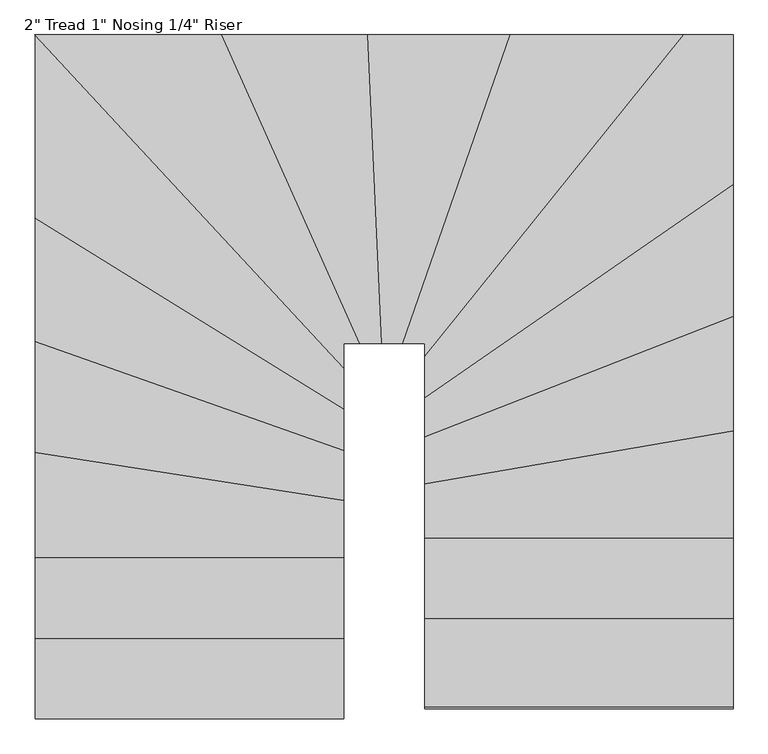
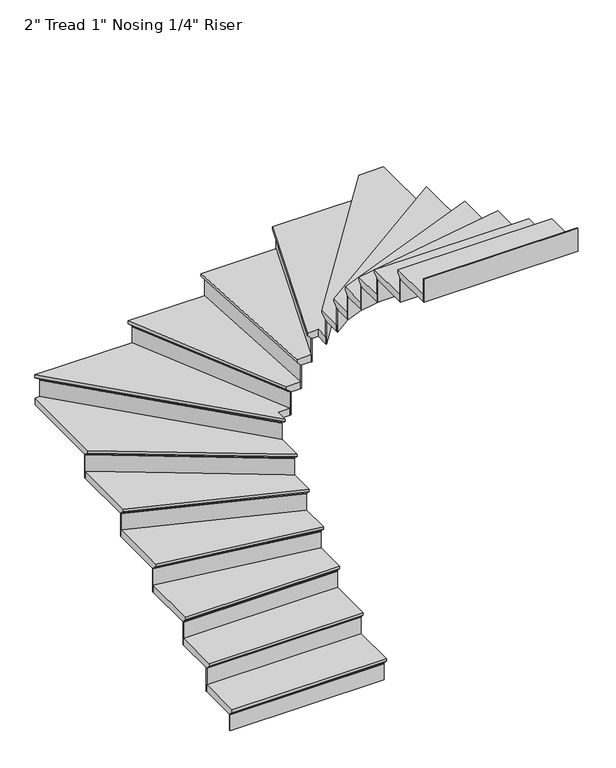
"""IFC4 building model written with IfcOpenShell, lengths in millimetres: stair flight geometry."""

from ifc_helpers import new_model, si_unit, origin, place, context, project, spatial, faceted_brep, source, transform, mapped, element, save


def stair_flight_3064df67(model_context):
    return source(origin(), model_context, "Body", "Brep", [
        faceted_brep([(-7275.2611447, 8794.085558, 319.6166667), (-7275.2611447, 8794.085558, 338.6666667), (-8342.0611447, 8794.085558, 338.6666667), (-8342.0611447, 8794.085558, 319.6166667), (-7275.2611447, 8819.485558, 294.2166667), (-8342.0611447, 8819.485558, 294.2166667), (-7275.2611447, 9098.885558, 338.6666667), (-8342.0611447, 9098.885558, 338.6666667), (-8342.0611447, 8819.485558, 287.8666667), (-8342.0611447, 9098.885558, 287.8666667), (-7275.2611447, 9098.885558, 287.8666667), (-7275.2611447, 8819.485558, 287.8666667)], [[[0, 1, 2, 3]], [[4, 0, 3, 5]], [[2, 1, 6, 7]], [[8, 9, 10, 11]], [[2, 7, 9, 8, 5, 3]], [[8, 11, 4, 5]], [[6, 1, 0, 4, 11, 10]], [[7, 6, 10, 9]]]),
        faceted_brep([(-7275.2611447, 8819.485558, 287.8666667), (-7275.2611447, 8819.485558, 169.3333333), (-7275.2611447, 8825.835558, 169.3333333), (-7275.2611447, 8825.835558, 287.8666667), (-8342.0611447, 8819.485558, 287.8666667), (-8342.0611447, 8825.835558, 287.8666667), (-8342.0611447, 8825.835558, 169.3333333), (-8342.0611447, 8819.485558, 169.3333333)], [[[0, 1, 2, 3]], [[4, 5, 6, 7]], [[1, 0, 4, 7]], [[2, 1, 7, 6]], [[3, 2, 6, 5]], [[0, 3, 5, 4]]]),
        faceted_brep([(-7275.2611447, 9098.885558, 457.2), (-7275.2611447, 9098.885558, 287.8666667), (-7275.2611447, 9105.235558, 287.8666667), (-7275.2611447, 9105.235558, 457.2), (-8342.0611447, 9098.885558, 457.2), (-8342.0611447, 9105.235558, 457.2), (-8342.0611447, 9105.235558, 287.8666667), (-8342.0611447, 9098.885558, 287.8666667)], [[[0, 1, 2, 3]], [[4, 5, 6, 7]], [[1, 0, 4, 7]], [[2, 1, 7, 6]], [[3, 2, 6, 5]], [[0, 3, 5, 4]]]),
        faceted_brep([(-8342.0611447, 9073.485558, 508.0), (-7275.2611447, 9073.485558, 508.0), (-7275.2611447, 9378.285558, 508.0), (-8342.0611447, 9378.285558, 508.0), (-8342.0611447, 9098.885558, 457.2), (-8342.0611447, 9378.285558, 457.2), (-7275.2611447, 9378.285558, 457.2), (-7275.2611447, 9098.885558, 457.2), (-8342.0611447, 9098.885558, 463.55), (-8342.0611447, 9073.485558, 488.95), (-7275.2611447, 9098.885558, 463.55), (-7275.2611447, 9073.485558, 488.95)], [[[0, 1, 2, 3]], [[4, 5, 6, 7]], [[0, 3, 5, 4, 8, 9]], [[4, 7, 10, 8]], [[2, 1, 11, 10, 7, 6]], [[3, 2, 6, 5]], [[11, 1, 0, 9]], [[10, 11, 9, 8]]]),
        faceted_brep([(-7275.2611447, 9378.285558, 626.5333333), (-7275.2611447, 9378.285558, 457.2), (-7275.2611447, 9384.635558, 457.2), (-7275.2611447, 9384.635558, 626.5333333), (-8342.0611447, 9378.285558, 626.5333333), (-8342.0611447, 9384.635558, 626.5333333), (-8342.0611447, 9384.635558, 457.2), (-8342.0611447, 9378.285558, 457.2)], [[[0, 1, 2, 3]], [[4, 5, 6, 7]], [[1, 0, 4, 7]], [[2, 1, 7, 6]], [[3, 2, 6, 5]], [[0, 3, 5, 4]]]),
        faceted_brep([(-8342.0611447, 9352.885558, 677.3333333), (-7275.2611447, 9352.885558, 677.3333333), (-7275.2611447, 9575.3066184, 677.3333333), (-8342.0611447, 9740.6711878, 677.3333333), (-8342.0611447, 9378.285558, 626.5333333), (-8342.0611447, 9740.6711878, 626.5333333), (-7275.2611447, 9575.3066184, 626.5333333), (-7275.2611447, 9378.285558, 626.5333333), (-8342.0611447, 9378.285558, 632.8833333), (-8342.0611447, 9352.885558, 658.2833333), (-7275.2611447, 9378.285558, 632.8833333), (-7275.2611447, 9352.885558, 658.2833333)], [[[0, 1, 2, 3]], [[4, 5, 6, 7]], [[0, 3, 5, 4, 8, 9]], [[4, 7, 10, 8]], [[2, 1, 11, 10, 7, 6]], [[3, 2, 6, 5]], [[11, 1, 0, 9]], [[10, 11, 9, 8]]]),
        faceted_brep([(-7275.2611447, 9575.3066184, 795.8666667), (-7275.2611447, 9575.3066184, 626.5333333), (-7275.2611447, 9581.7324547, 626.5333333), (-7275.2611447, 9581.7324547, 795.8666667), (-8342.0611447, 9740.6711878, 795.8666667), (-8342.0611447, 9747.0970241, 795.8666667), (-8342.0611447, 9747.0970241, 626.5333333), (-8342.0611447, 9740.6711878, 626.5333333)], [[[0, 1, 2, 3]], [[4, 5, 6, 7]], [[1, 0, 4, 7]], [[2, 1, 7, 6]], [[3, 2, 6, 5]], [[0, 3, 5, 4]]]),
        faceted_brep([(-8342.0611447, 9714.9678427, 846.6666667), (-7275.2611447, 9549.6032733, 846.6666667), (-7275.2611447, 9750.1745044, 846.6666667), (-8342.0611447, 10127.0738414, 846.6666667), (-8342.0611447, 9740.6711878, 795.8666667), (-8342.0611447, 10127.0738414, 795.8666667), (-7275.2611447, 9750.1745044, 795.8666667), (-7275.2611447, 9575.3066184, 795.8666667), (-8342.0611447, 9740.6711878, 802.2166667), (-8342.0611447, 9714.9678427, 827.6166667), (-7275.2611447, 9575.3066184, 802.2166667), (-7275.2611447, 9549.6032733, 827.6166667)], [[[0, 1, 2, 3]], [[4, 5, 6, 7]], [[0, 3, 5, 4, 8, 9]], [[4, 7, 10, 8]], [[2, 1, 11, 10, 7, 6]], [[3, 2, 6, 5]], [[11, 1, 0, 9]], [[10, 11, 9, 8]]]),
        faceted_brep([(-7275.2611447, 9750.1745044, 965.2), (-7275.2611447, 9750.1745044, 795.8666667), (-7275.2611447, 9756.9091582, 795.8666667), (-7275.2611447, 9756.9091582, 965.2), (-8342.0611447, 10127.0738414, 965.2), (-8342.0611447, 10133.8084951, 965.2), (-8342.0611447, 10133.8084951, 795.8666667), (-8342.0611447, 10127.0738414, 795.8666667)], [[[0, 1, 2, 3]], [[4, 5, 6, 7]], [[1, 0, 4, 7]], [[2, 1, 7, 6]], [[3, 2, 6, 5]], [[0, 3, 5, 4]]]),
        faceted_brep([(-8342.0611447, 10100.1352265, 1016.0), (-7275.2611447, 9723.2358895, 1016.0), (-7275.2611447, 9895.7459914, 1016.0), (-8342.0611447, 10557.0969884, 1016.0), (-8342.0611447, 10127.0738414, 965.2), (-8342.0611447, 10557.0969884, 965.2), (-7275.2611447, 9895.7459914, 965.2), (-7275.2611447, 9750.1745044, 965.2), (-8342.0611447, 10127.0738414, 971.55), (-8342.0611447, 10100.1352265, 996.95), (-7275.2611447, 9750.1745044, 971.55), (-7275.2611447, 9723.2358895, 996.95)], [[[0, 1, 2, 3]], [[4, 5, 6, 7]], [[0, 3, 5, 4, 8, 9]], [[4, 7, 10, 8]], [[2, 1, 11, 10, 7, 6]], [[3, 2, 6, 5]], [[11, 1, 0, 9]], [[10, 11, 9, 8]]]),
        faceted_brep([(-7275.2611447, 9895.7459914, 1134.5333333), (-7275.2611447, 9895.7459914, 965.2), (-7275.2611447, 9903.2172311, 965.2), (-7275.2611447, 9903.2172311, 1134.5333333), (-8342.0611447, 10557.0969884, 1134.5333333), (-8342.0611447, 10564.5682281, 1134.5333333), (-8342.0611447, 10564.5682281, 965.2), (-8342.0611447, 10557.0969884, 965.2)], [[[0, 1, 2, 3]], [[4, 5, 6, 7]], [[1, 0, 4, 7]], [[2, 1, 7, 6]], [[3, 2, 6, 5]], [[0, 3, 5, 4]]]),
        faceted_brep([(-8308.3760787, 11160.0172498, 1185.3333333), (-8342.0611447, 11160.0172498, 1185.3333333), (-8342.0611447, 10527.2120297, 1185.3333333), (-7275.2611447, 9865.8610326, 1185.3333333), (-7275.2611447, 10045.0066505, 1185.3333333), (-8342.0611447, 11160.0172498, 1134.5333333), (-8308.3760787, 11160.0172498, 1134.5333333), (-7275.2611447, 10045.0066505, 1134.5333333), (-7275.2611447, 9895.7459914, 1134.5333333), (-8342.0611447, 10557.0969884, 1134.5333333), (-7275.2611447, 9895.7459914, 1140.8833333), (-8342.0611447, 10557.0969884, 1140.8833333), (-7275.2611447, 9865.8610326, 1166.2833333), (-8342.0611447, 10527.2120297, 1166.2833333)], [[[0, 1, 2, 3, 4]], [[5, 6, 7, 8, 9]], [[1, 0, 6, 5]], [[9, 8, 10, 11]], [[4, 3, 12, 10, 8, 7]], [[0, 4, 7, 6]], [[12, 3, 2, 13]], [[10, 12, 13, 11]], [[2, 1, 5, 9, 11, 13]]]),
        faceted_brep([(-7275.2611447, 10045.0066505, 1303.8666667), (-7275.2611447, 10045.0066505, 1134.5333333), (-7275.2611447, 10054.3496243, 1134.5333333), (-7275.2611447, 10054.3496243, 1303.8666667), (-8308.3760787, 11160.0172498, 1303.8666667), (-8299.7193307, 11160.0172498, 1303.8666667), (-8299.7193307, 11160.0172498, 1134.5333333), (-8308.3760787, 11160.0172498, 1134.5333333)], [[[0, 1, 2, 3]], [[4, 5, 6, 7]], [[1, 0, 4, 7]], [[2, 1, 7, 6]], [[3, 2, 6, 5]], [[0, 3, 5, 4]]]),
        faceted_brep([(-8343.0030706, 11160.0172498, 1354.6666667), (-7275.2611447, 10007.6347554, 1354.6666667), (-7275.2611447, 10093.2172498, 1354.6666667), (-7192.6344871, 10093.2172498, 1354.6666667), (-7669.6752678, 11160.0172498, 1354.6666667), (-8308.3760787, 11160.0172498, 1303.8666667), (-7669.6752678, 11160.0172498, 1303.8666667), (-7192.6344871, 10093.2172498, 1303.8666667), (-7275.2611447, 10093.2172498, 1303.8666667), (-7275.2611447, 10045.0066505, 1303.8666667), (-8308.3760787, 11160.0172498, 1310.2166667), (-8343.0030706, 11160.0172498, 1335.6166667), (-7275.2611447, 10045.0066505, 1310.2166667), (-7275.2611447, 10007.6347554, 1335.6166667)], [[[0, 1, 2, 3, 4]], [[5, 6, 7, 8, 9]], [[0, 4, 6, 5, 10, 11]], [[5, 9, 12, 10]], [[2, 1, 13, 12, 9, 8]], [[3, 2, 8, 7]], [[4, 3, 7, 6]], [[13, 1, 0, 11]], [[12, 13, 11, 10]]]),
        faceted_brep([(-7192.6344871, 10093.2172498, 1473.2), (-7192.6344871, 10093.2172498, 1303.8666667), (-7185.6785241, 10093.2172498, 1303.8666667), (-7185.6785241, 10093.2172498, 1473.2), (-7669.6752678, 11160.0172498, 1473.2), (-7662.7193048, 11160.0172498, 1473.2), (-7662.7193048, 11160.0172498, 1303.8666667), (-7669.6752678, 11160.0172498, 1303.8666667)], [[[0, 1, 2, 3]], [[4, 5, 6, 7]], [[1, 0, 4, 7]], [[2, 1, 7, 6]], [[3, 2, 6, 5]], [[0, 3, 5, 4]]]),
        faceted_brep([(-7697.49912, 11160.0172498, 1524.0), (-7220.4583393, 10093.2172498, 1524.0), (-7118.6029726, 10093.2172498, 1524.0), (-7167.3410541, 11160.0172498, 1524.0), (-7669.6752678, 11160.0172498, 1473.2), (-7167.3410541, 11160.0172498, 1473.2), (-7118.6029726, 10093.2172498, 1473.2), (-7192.6344871, 10093.2172498, 1473.2), (-7669.6752678, 11160.0172498, 1479.55), (-7697.49912, 11160.0172498, 1504.95), (-7192.6344871, 10093.2172498, 1479.55), (-7220.4583393, 10093.2172498, 1504.95)], [[[0, 1, 2, 3]], [[4, 5, 6, 7]], [[0, 3, 5, 4, 8, 9]], [[4, 7, 10, 8]], [[3, 2, 6, 5]], [[11, 1, 0, 9]], [[10, 11, 9, 8]], [[2, 1, 11, 10, 7, 6]]]),
        faceted_brep([(-7118.6029726, 10093.2172498, 1642.5333333), (-7118.6029726, 10093.2172498, 1473.2), (-7112.2463491, 10093.2172498, 1473.2), (-7112.2463491, 10093.2172498, 1642.5333333), (-7167.3410541, 11160.0172498, 1642.5333333), (-7160.9844306, 11160.0172498, 1642.5333333), (-7160.9844306, 11160.0172498, 1473.2), (-7167.3410541, 11160.0172498, 1473.2)], [[[0, 1, 2, 3]], [[4, 5, 6, 7]], [[1, 0, 4, 7]], [[2, 1, 7, 6]], [[3, 2, 6, 5]], [[0, 3, 5, 4]]]),
        faceted_brep([(-7192.7675482, 11160.0172498, 1693.3333333), (-7144.0294667, 10093.2172498, 1693.3333333), (-7045.1202005, 10093.2172498, 1693.3333333), (-6671.9374808, 11160.0172498, 1693.3333333), (-7167.3410541, 11160.0172498, 1642.5333333), (-6671.9374808, 11160.0172498, 1642.5333333), (-7045.1202005, 10093.2172498, 1642.5333333), (-7118.6029726, 10093.2172498, 1642.5333333), (-7167.3410541, 11160.0172498, 1648.8833333), (-7192.7675482, 11160.0172498, 1674.2833333), (-7118.6029726, 10093.2172498, 1648.8833333), (-7144.0294667, 10093.2172498, 1674.2833333)], [[[0, 1, 2, 3]], [[4, 5, 6, 7]], [[0, 3, 5, 4, 8, 9]], [[4, 7, 10, 8]], [[2, 1, 11, 10, 7, 6]], [[3, 2, 6, 5]], [[11, 1, 0, 9]], [[10, 11, 9, 8]]]),
        faceted_brep([(-7045.1202005, 10093.2172498, 1811.8666667), (-7045.1202005, 10093.2172498, 1642.5333333), (-7038.3928839, 10093.2172498, 1642.5333333), (-7038.3928839, 10093.2172498, 1811.8666667), (-6671.9374808, 11160.0172498, 1811.8666667), (-6665.2101642, 11160.0172498, 1811.8666667), (-6665.2101642, 11160.0172498, 1642.5333333), (-6671.9374808, 11160.0172498, 1642.5333333)], [[[0, 1, 2, 3]], [[4, 5, 6, 7]], [[1, 0, 4, 7]], [[2, 1, 7, 6]], [[3, 2, 6, 5]], [[0, 3, 5, 4]]]),
        faceted_brep([(-6698.8467469, 11160.0172498, 1862.6666667), (-7072.0294667, 10093.2172498, 1862.6666667), (-6995.8611447, 10093.2172498, 1862.6666667), (-6995.8611447, 10007.4990501, 1862.6666667), (-6067.5072178, 11160.0172498, 1862.6666667), (-6671.9374808, 11160.0172498, 1811.8666667), (-6067.5072178, 11160.0172498, 1811.8666667), (-6995.8611447, 10007.4990501, 1811.8666667), (-6995.8611447, 10093.2172498, 1811.8666667), (-7045.1202005, 10093.2172498, 1811.8666667), (-6671.9374808, 11160.0172498, 1818.2166667), (-6698.8467469, 11160.0172498, 1843.6166667), (-7045.1202005, 10093.2172498, 1818.2166667), (-7072.0294667, 10093.2172498, 1843.6166667)], [[[0, 1, 2, 3, 4]], [[5, 6, 7, 8, 9]], [[0, 4, 6, 5, 10, 11]], [[5, 9, 12, 10]], [[2, 1, 13, 12, 9, 8]], [[3, 2, 8, 7]], [[4, 3, 7, 6]], [[13, 1, 0, 11]], [[12, 13, 11, 10]]]),
        faceted_brep([(-6995.8611447, 10007.4990501, 1981.2), (-6995.8611447, 10007.4990501, 1811.8666667), (-6995.8611447, 9997.3763585, 1811.8666667), (-6995.8611447, 9997.3763585, 1981.2), (-6067.5072178, 11160.0172498, 1981.2), (-6059.3533852, 11160.0172498, 1981.2), (-6059.3533852, 11160.0172498, 1811.8666667), (-6067.5072178, 11160.0172498, 1811.8666667)], [[[0, 1, 2, 3]], [[4, 5, 6, 7]], [[1, 0, 4, 7]], [[2, 1, 7, 6]], [[3, 2, 6, 5]], [[0, 3, 5, 4]]]),
        faceted_brep([(-5929.0611447, 10611.3875661, 2032.0), (-5929.0611447, 11160.0172498, 2032.0), (-6100.1225484, 11160.0172498, 2032.0), (-6995.8611447, 10047.9898167, 2032.0), (-6995.8611447, 9873.2783158, 2032.0), (-5929.0611447, 11160.0172498, 1981.2), (-5929.0611447, 10611.3875661, 1981.2), (-6995.8611447, 9873.2783158, 1981.2), (-6995.8611447, 10007.4990501, 1981.2), (-6067.5072178, 11160.0172498, 1981.2), (-6067.5072178, 11160.0172498, 1987.55), (-6100.1225484, 11160.0172498, 2012.95), (-6995.8611447, 10007.4990501, 1987.55), (-6995.8611447, 10047.9898167, 2012.95)], [[[0, 1, 2, 3, 4]], [[5, 6, 7, 8, 9]], [[1, 0, 6, 5]], [[2, 1, 5, 9, 10, 11]], [[9, 8, 12, 10]], [[4, 3, 13, 12, 8, 7]], [[0, 4, 7, 6]], [[13, 3, 2, 11]], [[12, 13, 11, 10]]]),
        faceted_brep([(-6995.8611447, 9873.2783158, 2150.5333333), (-6995.8611447, 9873.2783158, 1981.2), (-6995.8611447, 9865.5565668, 1981.2), (-6995.8611447, 9865.5565668, 2150.5333333), (-5929.0611447, 10611.3875661, 2150.5333333), (-5929.0611447, 10603.6658171, 2150.5333333), (-5929.0611447, 10603.6658171, 1981.2), (-5929.0611447, 10611.3875661, 1981.2)], [[[0, 1, 2, 3]], [[4, 5, 6, 7]], [[1, 0, 4, 7]], [[2, 1, 7, 6]], [[3, 2, 6, 5]], [[0, 3, 5, 4]]]),
        faceted_brep([(-5929.0611447, 10642.2745621, 2201.3333333), (-6995.8611447, 9904.1653118, 2201.3333333), (-6995.8611447, 9741.7204172, 2201.3333333), (-5929.0611447, 10158.6104329, 2201.3333333), (-5929.0611447, 10611.3875661, 2150.5333333), (-5929.0611447, 10158.6104329, 2150.5333333), (-6995.8611447, 9741.7204172, 2150.5333333), (-6995.8611447, 9873.2783158, 2150.5333333), (-5929.0611447, 10611.3875661, 2156.8833333), (-5929.0611447, 10642.2745621, 2182.2833333), (-6995.8611447, 9873.2783158, 2156.8833333), (-6995.8611447, 9904.1653118, 2182.2833333)], [[[0, 1, 2, 3]], [[4, 5, 6, 7]], [[0, 3, 5, 4, 8, 9]], [[4, 7, 10, 8]], [[2, 1, 11, 10, 7, 6]], [[3, 2, 6, 5]], [[11, 1, 0, 9]], [[10, 11, 9, 8]]]),
        faceted_brep([(-6995.8611447, 9741.7204172, 2319.8666667), (-6995.8611447, 9741.7204172, 2150.5333333), (-6995.8611447, 9734.9027722, 2150.5333333), (-6995.8611447, 9734.9027722, 2319.8666667), (-5929.0611447, 10158.6104329, 2319.8666667), (-5929.0611447, 10151.7927879, 2319.8666667), (-5929.0611447, 10151.7927879, 2150.5333333), (-5929.0611447, 10158.6104329, 2150.5333333)], [[[0, 1, 2, 3]], [[4, 5, 6, 7]], [[1, 0, 4, 7]], [[2, 1, 7, 6]], [[3, 2, 6, 5]], [[0, 3, 5, 4]]]),
        faceted_brep([(-5929.0611447, 10185.881013, 2370.6666667), (-6995.8611447, 9768.9909973, 2370.6666667), (-6995.8611447, 9580.5364125, 2370.6666667), (-5929.0611447, 9763.9899323, 2370.6666667), (-5929.0611447, 10158.6104329, 2319.8666667), (-5929.0611447, 9763.9899323, 2319.8666667), (-6995.8611447, 9580.5364125, 2319.8666667), (-6995.8611447, 9741.7204172, 2319.8666667), (-5929.0611447, 10158.6104329, 2326.2166667), (-5929.0611447, 10185.881013, 2351.6166667), (-6995.8611447, 9741.7204172, 2326.2166667), (-6995.8611447, 9768.9909973, 2351.6166667)], [[[0, 1, 2, 3]], [[4, 5, 6, 7]], [[0, 3, 5, 4, 8, 9]], [[4, 7, 10, 8]], [[2, 1, 11, 10, 7, 6]], [[3, 2, 6, 5]], [[11, 1, 0, 9]], [[10, 11, 9, 8]]]),
        faceted_brep([(-6995.8611447, 9580.5364125, 2489.2), (-6995.8611447, 9580.5364125, 2319.8666667), (-6995.8611447, 9574.0932043, 2319.8666667), (-6995.8611447, 9574.0932043, 2489.2), (-5929.0611447, 9763.9899323, 2489.2), (-5929.0611447, 9757.5467241, 2489.2), (-5929.0611447, 9757.5467241, 2319.8666667), (-5929.0611447, 9763.9899323, 2319.8666667)], [[[0, 1, 2, 3]], [[4, 5, 6, 7]], [[1, 0, 4, 7]], [[2, 1, 7, 6]], [[3, 2, 6, 5]], [[0, 3, 5, 4]]]),
        faceted_brep([(-5929.0611447, 9789.762765, 2540.0), (-6995.8611447, 9606.3092452, 2540.0), (-6995.8611447, 9393.2360051, 2540.0), (-5929.0611447, 9393.2360051, 2540.0), (-5929.0611447, 9763.9899323, 2489.2), (-5929.0611447, 9393.2360051, 2489.2), (-6995.8611447, 9393.2360051, 2489.2), (-6995.8611447, 9580.5364125, 2489.2), (-5929.0611447, 9763.9899323, 2495.55), (-5929.0611447, 9789.762765, 2520.95), (-6995.8611447, 9580.5364125, 2495.55), (-6995.8611447, 9606.3092452, 2520.95)], [[[0, 1, 2, 3]], [[4, 5, 6, 7]], [[0, 3, 5, 4, 8, 9]], [[4, 7, 10, 8]], [[2, 1, 11, 10, 7, 6]], [[3, 2, 6, 5]], [[11, 1, 0, 9]], [[10, 11, 9, 8]]]),
        faceted_brep([(-6995.8611447, 9393.2360051, 2658.5333333), (-6995.8611447, 9393.2360051, 2489.2), (-6995.8611447, 9386.8860051, 2489.2), (-6995.8611447, 9386.8860051, 2658.5333333), (-5929.0611447, 9393.2360051, 2658.5333333), (-5929.0611447, 9386.8860051, 2658.5333333), (-5929.0611447, 9386.8860051, 2489.2), (-5929.0611447, 9393.2360051, 2489.2)], [[[0, 1, 2, 3]], [[4, 5, 6, 7]], [[1, 0, 4, 7]], [[2, 1, 7, 6]], [[3, 2, 6, 5]], [[0, 3, 5, 4]]]),
        faceted_brep([(-5929.0611447, 9418.6360051, 2709.3333333), (-6995.8611447, 9418.6360051, 2709.3333333), (-6995.8611447, 9113.8360051, 2709.3333333), (-5929.0611447, 9113.8360051, 2709.3333333), (-5929.0611447, 9393.2360051, 2658.5333333), (-5929.0611447, 9113.8360051, 2658.5333333), (-6995.8611447, 9113.8360051, 2658.5333333), (-6995.8611447, 9393.2360051, 2658.5333333), (-5929.0611447, 9393.2360051, 2664.8833333), (-5929.0611447, 9418.6360051, 2690.2833333), (-6995.8611447, 9393.2360051, 2664.8833333), (-6995.8611447, 9418.6360051, 2690.2833333)], [[[0, 1, 2, 3]], [[4, 5, 6, 7]], [[0, 3, 5, 4, 8, 9]], [[4, 7, 10, 8]], [[2, 1, 11, 10, 7, 6]], [[3, 2, 6, 5]], [[11, 1, 0, 9]], [[10, 11, 9, 8]]]),
        faceted_brep([(-6995.8611447, 9113.8360051, 2827.8666667), (-6995.8611447, 9113.8360051, 2658.5333333), (-6995.8611447, 9107.4860051, 2658.5333333), (-6995.8611447, 9107.4860051, 2827.8666667), (-5929.0611447, 9113.8360051, 2827.8666667), (-5929.0611447, 9107.4860051, 2827.8666667), (-5929.0611447, 9107.4860051, 2658.5333333), (-5929.0611447, 9113.8360051, 2658.5333333)], [[[0, 1, 2, 3]], [[4, 5, 6, 7]], [[1, 0, 4, 7]], [[2, 1, 7, 6]], [[3, 2, 6, 5]], [[0, 3, 5, 4]]]),
        faceted_brep([(-6995.8611447, 8834.4360051, 2997.2), (-6995.8611447, 8834.4360051, 2827.8666667), (-6995.8611447, 8828.0860051, 2827.8666667), (-6995.8611447, 8828.0860051, 2997.2), (-5929.0611447, 8834.4360051, 2997.2), (-5929.0611447, 8828.0860051, 2997.2), (-5929.0611447, 8828.0860051, 2827.8666667), (-5929.0611447, 8834.4360051, 2827.8666667)], [[[0, 1, 2, 3]], [[4, 5, 6, 7]], [[1, 0, 4, 7]], [[2, 1, 7, 6]], [[3, 2, 6, 5]], [[0, 3, 5, 4]]]),
        faceted_brep([(-5929.0611447, 9139.2360051, 2878.6666667), (-6995.8611447, 9139.2360051, 2878.6666667), (-6995.8611447, 8834.4360051, 2878.6666667), (-5929.0611447, 8834.4360051, 2878.6666667), (-5929.0611447, 9113.8360051, 2827.8666667), (-5929.0611447, 8834.4360051, 2827.8666667), (-6995.8611447, 8834.4360051, 2827.8666667), (-6995.8611447, 9113.8360051, 2827.8666667), (-5929.0611447, 9113.8360051, 2834.2166667), (-5929.0611447, 9139.2360051, 2859.6166667), (-6995.8611447, 9113.8360051, 2834.2166667), (-6995.8611447, 9139.2360051, 2859.6166667)], [[[0, 1, 2, 3]], [[4, 5, 6, 7]], [[0, 3, 5, 4, 8, 9]], [[4, 7, 10, 8]], [[2, 1, 11, 10, 7, 6]], [[3, 2, 6, 5]], [[11, 1, 0, 9]], [[10, 11, 9, 8]]]),
    ])


if __name__ == "__main__":
    model = new_model("IFC4")
    model_context = context("Model", 3, world=origin())
    ifc_project = project(units=[si_unit("LENGTHUNIT", "METRE", prefix="MILLI")], contexts=[model_context])
    site = spatial("IfcSite", under=ifc_project)
    building = spatial("IfcBuilding", under=site)
    placement = place(None, origin())
    stair_flight_shape = stair_flight_3064df67(model_context)
    element("IfcStairFlight", 1, ObjectType="2\" Tread 1\" Nosing 1/4\" Riser", at=placement, inside=building, context=model_context, shape_type="MappedRepresentation", body=[
        mapped(stair_flight_shape, transform((0.0, 0.0, 0.0), x_axis=(1.0, 0.0, 0.0), y_axis=(0.0, 1.0, 0.0), z_axis=(0.0, 0.0, 1.0))),
    ])
    save(model, "model.ifc")
